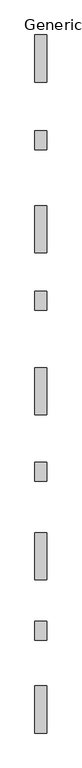
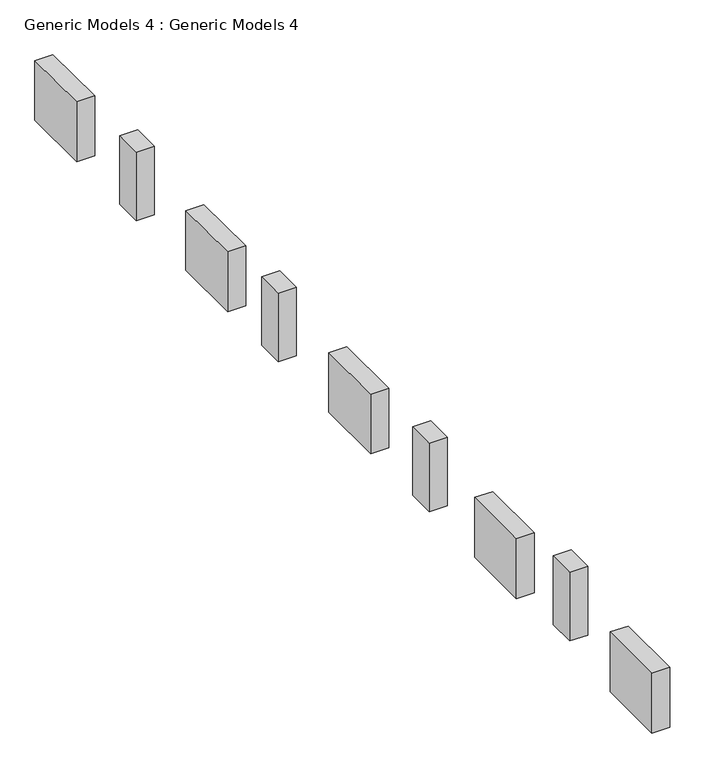
"""IFC4 building model written with IfcOpenShell, lengths in millimetres: proxy geometry, Generic Models 4 : Generic Models 4."""

from ifc_helpers import new_model, si_unit, frame, origin, place, context, project, spatial, polyline, outline, extrude, source, transform, mapped, element, save


def generic_models_4_generic_models_4_94af110e(model_context):
    return source(origin(), model_context, "Body", "SweptSolid", [
        extrude(outline(polyline([(-7399.9793212, 8285.5730531), (-7399.9793212, 9504.7730531), (-7095.1793212, 9504.7730531), (-7095.1793212, 8285.5730531), (-7399.9793212, 8285.5730531)])), frame((0.0, 0.0, 188.9807159), z_axis=(0.0, 0.0, 1.0), x_axis=(1.0, 0.0, 0.0)), (0.0, 0.0, 1.0), 1066.8),
        extrude(outline(polyline([(-7399.9793212, 6540.160923), (-7399.9793212, 7024.8568889), (-7095.1793212, 7024.8568889), (-7095.1793212, 6540.160923), (-7399.9793212, 6540.160923)])), frame((0.0, 0.0, 188.9807159), z_axis=(0.0, 0.0, 1.0), x_axis=(1.0, 0.0, 0.0)), (0.0, 0.0, 1.0), 1228.6150263),
        extrude(outline(polyline([(-7399.9793212, 3865.9730531), (-7399.9793212, 5085.1730531), (-7095.1793212, 5085.1730531), (-7095.1793212, 3865.9730531), (-7399.9793212, 3865.9730531)])), frame((0.0, 0.0, 188.9807159), z_axis=(0.0, 0.0, 1.0), x_axis=(1.0, 0.0, 0.0)), (0.0, 0.0, 1.0), 1066.8),
        extrude(outline(polyline([(-7399.9793212, -319.0564015), (-7399.9793212, 900.1435985), (-7095.1793212, 900.1435985), (-7095.1793212, -319.0564015), (-7399.9793212, -319.0564015)])), frame((0.0, 0.0, 188.9807159), z_axis=(0.0, 0.0, 1.0), x_axis=(1.0, 0.0, 0.0)), (0.0, 0.0, 1.0), 1066.8),
        extrude(outline(polyline([(-7399.9793212, -4586.2564015), (-7399.9793212, -3367.0564015), (-7095.1793212, -3367.0564015), (-7095.1793212, -4586.2564015), (-7399.9793212, -4586.2564015)])), frame((0.0, 0.0, 188.9807159), z_axis=(0.0, 0.0, 1.0), x_axis=(1.0, 0.0, 0.0)), (0.0, 0.0, 1.0), 1066.8),
        extrude(outline(polyline([(-7399.9793212, -8548.6564015), (-7399.9793212, -7329.4564015), (-7095.1793212, -7329.4564015), (-7095.1793212, -8548.6564015), (-7399.9793212, -8548.6564015)])), frame((0.0, 0.0, 188.9807159), z_axis=(0.0, 0.0, 1.0), x_axis=(1.0, 0.0, 0.0)), (0.0, 0.0, 1.0), 1066.8),
        extrude(outline(polyline([(-7399.9793212, 2387.260923), (-7399.9793212, 2871.9568889), (-7095.1793212, 2871.9568889), (-7095.1793212, 2387.260923), (-7399.9793212, 2387.260923)])), frame((0.0, 0.0, 188.9807159), z_axis=(0.0, 0.0, 1.0), x_axis=(1.0, 0.0, 0.0)), (0.0, 0.0, 1.0), 1228.6150263),
        extrude(outline(polyline([(-7399.9793212, -2032.339077), (-7399.9793212, -1547.6431111), (-7095.1793212, -1547.6431111), (-7095.1793212, -2032.339077), (-7399.9793212, -2032.339077)])), frame((0.0, 0.0, 188.9807159), z_axis=(0.0, 0.0, 1.0), x_axis=(1.0, 0.0, 0.0)), (0.0, 0.0, 1.0), 1228.6150263),
        extrude(outline(polyline([(-7399.9793212, -6147.139077), (-7399.9793212, -5662.4431111), (-7095.1793212, -5662.4431111), (-7095.1793212, -6147.139077), (-7399.9793212, -6147.139077)])), frame((0.0, 0.0, 377.9614318), z_axis=(0.0, 0.0, 1.0), x_axis=(1.0, 0.0, 0.0)), (0.0, 0.0, 1.0), 1228.6150263),
    ])


if __name__ == "__main__":
    model = new_model("IFC4")
    model_context = context("Model", 3, world=origin())
    ifc_project = project(units=[si_unit("LENGTHUNIT", "METRE", prefix="MILLI")], contexts=[model_context])
    site = spatial("IfcSite", under=ifc_project)
    building = spatial("IfcBuilding", under=site)
    placement = place(None, origin())
    generic_models_4_generic_models_4_shape = generic_models_4_generic_models_4_94af110e(model_context)
    element("IfcBuildingElementProxy", 1, Name="Generic Models 4 : Generic Models 4", ObjectType="Generic Models 4 : Generic Models 4", at=placement, inside=building, context=model_context, shape_type="MappedRepresentation", body=[
        mapped(generic_models_4_generic_models_4_shape, transform((0.0, 0.0, 0.0), x_axis=(1.0, 0.0, 0.0), y_axis=(0.0, 1.0, 0.0), z_axis=(0.0, 0.0, 1.0))),
    ])
    save(model, "model.ifc")

# Revit data of these elements
# Element 1 (IfcBuildingElementProxy, "Generic Models 4 : Generic Models 4")
#   Materials on its faces: "Parking Stripe"
# Materials
#   "Parking Stripe": class "Paint", colour RGB 250 250 91, transparency 0, Cost = 0
